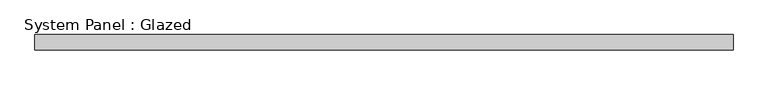
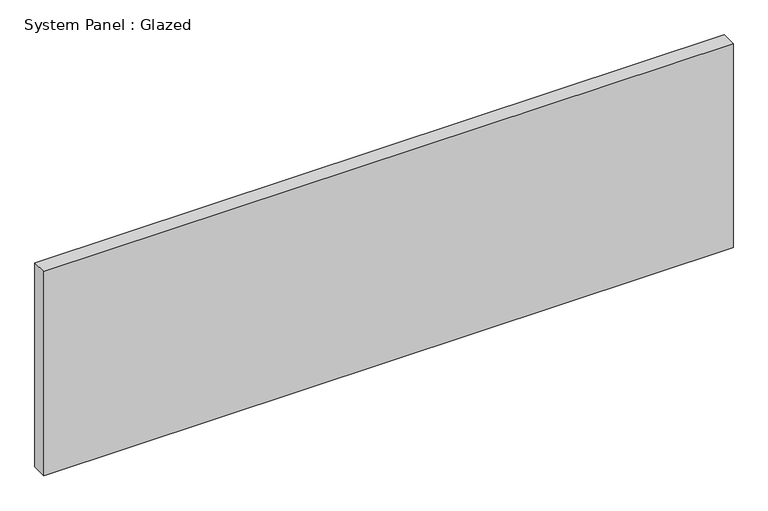
"""IFC4 building model written with IfcOpenShell, lengths in millimetres: plate geometry, System Panel : Glazed."""

from ifc_helpers import new_model, si_unit, origin, origin_with_axes, place, context, project, spatial, polyline, outline, extrude, source, transform, mapped, element, save


def system_panel_glazed_496eb5f8(model_context):
    return source(origin(), model_context, "Body", "SweptSolid", [
        extrude(outline(polyline([(577.85, 19.05), (-577.85, 19.05), (-577.85, 44.45), (577.85, 44.45), (577.85, 19.05)])), origin_with_axes(), (0.0, 0.0, 1.0), 361.95),
    ])


if __name__ == "__main__":
    model = new_model("IFC4")
    model_context = context("Model", 3, world=origin())
    ifc_project = project(units=[si_unit("LENGTHUNIT", "METRE", prefix="MILLI")], contexts=[model_context])
    site = spatial("IfcSite", under=ifc_project)
    building = spatial("IfcBuilding", under=site)
    placement = place(None, origin())
    system_panel_glazed_shape = system_panel_glazed_496eb5f8(model_context)
    element("IfcPlate", 1, ObjectType="System Panel : Glazed", at=placement, inside=building, context=model_context, shape_type="MappedRepresentation", body=[
        mapped(system_panel_glazed_shape, transform((0.0, 0.0, 0.0), x_axis=(1.0, 0.0, 0.0), y_axis=(0.0, 1.0, 0.0), z_axis=(0.0, 0.0, 1.0))),
    ])
    save(model, "model.ifc")

# Revit data of these elements
# Type "System Panel : Glazed"
#   Construction Type Id = "GSP4R"
#   Analytic Construction = "1/8 in Pilkington single glazing"
#   Visual Light Transmittance = 0.9
#   Solar Heat Gain Coefficient = 0.86
#   Heat Transfer Coefficient (U) = 1.18115 BTU/(h·ft²·°F)
#   Define Thermal Properties by = 1
# Element 1 (IfcPlate, "System Panel : Glazed")
#   Materials on its faces: "Glass"
# Materials
#   "Glass": class "Glass", colour RGB 0 128 192, transparency 0.75, Description = "Soda Lime Glass", Cost = 0
